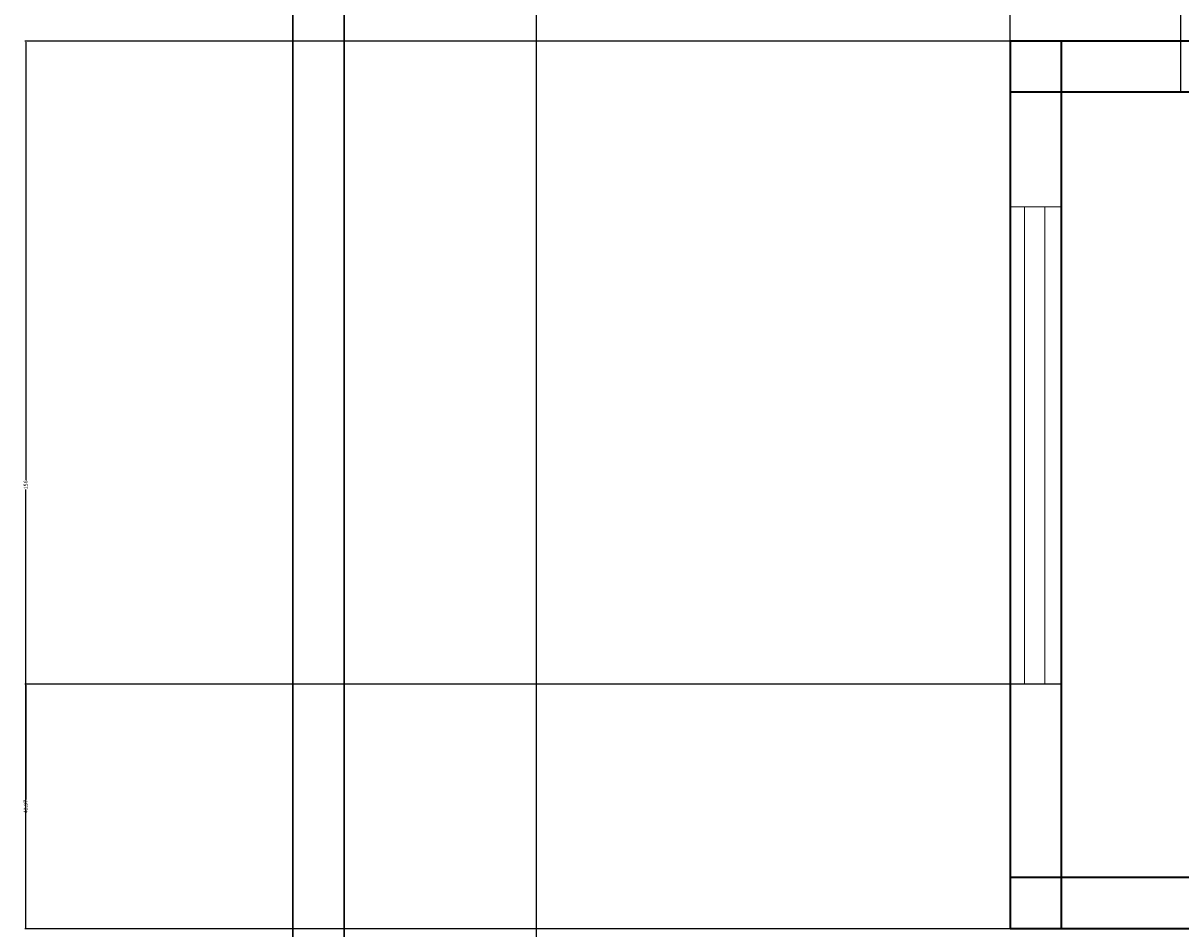
# Model space of a CAD drawing. Units: inches. Extents: x 867 to 1667, y -234 to 788.
# Tile 26 of 42: x 867 to 1071, y 258 to 417. Entities that reach past the tile are written whole.
import ezdxf

# ---------------------------------------------------------------- set-up
doc = ezdxf.new("R2010")
doc.units = ezdxf.units.IN
doc.header["$MEASUREMENT"] = 0
for name, color, linetype, lineweight in [('A-ANNO-DIMS', 2, 'Continuous', 18), ('A-Glaz', 92, 'Continuous', 18), ('A-Wall', 7, 'Continuous', 35), ('A-WALL-SITE', 8, 'Continuous', 30)]:
    doc.layers.add(name, color=color, linetype=linetype, lineweight=lineweight)
doc.styles.get("Standard").update_dxf_attribs({"font": 'arial.ttf'})
doc.dimstyles.get("Standard").update_dxf_attribs({"dimtxt": 0.6875, "dimasz": 0.18, "dimexe": 0.18, "dimexo": 0.0625, "dimgap": 0.09, "dimtad": 0, "dimdec": 4, "dimzin": 0, "dimdsep": 46, "dimlunit": 4, "dimtxsty": 'Standard', "dimcen": 0.09, "dimadec": 0, "dimazin": 0, "dimtfac": 1, "dimtdec": 4, "dimtofl": 0, "dimtmove": 0, "dimatfit": 3, "dimfxl": 1, "dimtolj": 1, "dimtzin": 0, "dimarcsym": 0})

# ---------------------------------------------------------------- blocks, each defined once
blk = doc.blocks.new('WIN-83_90IN')
for p, q in [((0, 83.9), (9, 83.9)), ((2.51, 83.9), (2.51, 0)), ((6.08, 0), (6.08, 83.9)), ((0, 0), (9, 0))]:
    blk.add_line(p, q)
blk = doc.blocks.new('*D28')
at = {"layer": 'A-ANNO-DIMS', "color": 0, "lineweight": -2, "transparency": 16777216}
for p, q in [((914.89, 623.55), (914.89, -233.54)), ((957.64, 623.55), (957.64, -233.54)), ((915.07, -233.36), (935, -233.36)), ((957.46, -233.36), (937.53, -233.36))]:
    blk.add_line(p, q, dxfattribs=at)
at = {"layer": 'A-ANNO-DIMS', "color": 0, "transparency": 16777216}
for points in [[(915.07, -233.33), (915.07, -233.39), (914.89, -233.36)], [(957.46, -233.33), (957.46, -233.39), (957.64, -233.36)]]:
    blk.add_solid(points, dxfattribs=at)
at = {"layer": 'Defpoints', "color": 0, "transparency": 16777216}
for p in [(914.89, 623.62), (957.64, 623.62), (914.89, -233.36)]:
    blk.add_point(p, dxfattribs=at)
at = {"layer": 'A-ANNO-DIMS', "color": 0, "transparency": 16777216, "insert": (936.26, -233.36), "char_height": 0.688, "attachment_point": 5}
blk.add_mtext('\\A1;42.75', dxfattribs=at)
blk = doc.blocks.new('*D35')
at = {"layer": 'A-ANNO-DIMS', "color": 0, "lineweight": -2, "transparency": 16777216}
for p, q in [((1040.89, 413.68), (1040.89, 787.75)), ((1041.07, 787.57), (1055.31, 787.57)), ((1070.71, 787.57), (1056.47, 787.57)), ((1070.89, 404.68), (1070.89, 787.75))]:
    blk.add_line(p, q, dxfattribs=at)
at = {"layer": 'A-ANNO-DIMS', "color": 0, "transparency": 16777216}
for points in [[(1041.07, 787.6), (1041.07, 787.54), (1040.89, 787.57)], [(1070.71, 787.6), (1070.71, 787.54), (1070.89, 787.57)]]:
    blk.add_solid(points, dxfattribs=at)
at = {"layer": 'Defpoints', "color": 0, "transparency": 16777216}
for p in [(1070.89, 787.57), (1040.89, 413.62), (1070.89, 404.62)]:
    blk.add_point(p, dxfattribs=at)
at = {"layer": 'A-ANNO-DIMS', "color": 0, "transparency": 16777216, "insert": (1055.89, 787.57), "char_height": 0.688, "attachment_point": 5}
blk.add_mtext('\\A1;30', dxfattribs=at)
blk = doc.blocks.new('*D39')
at = {"layer": 'A-ANNO-DIMS', "color": 0, "lineweight": -2, "transparency": 16777216}
for p, q in [((1040.82, 413.62), (867.76, 413.62)), ((867.94, 413.44), (867.94, 336.43)), ((867.94, 257.8), (867.94, 334.8)), ((1040.82, 257.62), (867.76, 257.62))]:
    blk.add_line(p, q, dxfattribs=at)
at = {"layer": 'A-ANNO-DIMS', "color": 0, "transparency": 16777216}
for points in [[(867.91, 413.44), (867.97, 413.44), (867.94, 413.62)], [(867.91, 257.8), (867.97, 257.8), (867.94, 257.62)]]:
    blk.add_solid(points, dxfattribs=at)
at = {"layer": 'Defpoints', "color": 0, "transparency": 16777216}
for p in [(867.94, 413.62), (1040.89, 413.62), (1040.89, 257.62)]:
    blk.add_point(p, dxfattribs=at)
at = {"layer": 'A-ANNO-DIMS', "color": 0, "transparency": 16777216, "insert": (867.94, 335.62), "char_height": 0.688, "attachment_point": 5, "rotation": 90}
blk.add_mtext('\\A1;156', dxfattribs=at)
blk = doc.blocks.new('*D56')
at = {"layer": 'A-ANNO-DIMS', "color": 0, "lineweight": -2, "transparency": 16777216}
for p, q in [((1049.82, 300.59), (867.76, 300.59)), ((867.94, 300.41), (867.94, 280.37)), ((867.94, 257.8), (867.94, 277.84)), ((1049.82, 257.62), (867.76, 257.62))]:
    blk.add_line(p, q, dxfattribs=at)
at = {"layer": 'A-ANNO-DIMS', "color": 0, "transparency": 16777216}
for points in [[(867.91, 300.41), (867.97, 300.41), (867.94, 300.59)], [(867.91, 257.8), (867.97, 257.8), (867.94, 257.62)]]:
    blk.add_solid(points, dxfattribs=at)
at = {"layer": 'Defpoints', "color": 0, "transparency": 16777216}
for p in [(867.94, 300.59), (1049.89, 300.59), (1049.89, 257.62)]:
    blk.add_point(p, dxfattribs=at)
at = {"layer": 'A-ANNO-DIMS', "color": 0, "transparency": 16777216, "insert": (867.94, 279.1), "char_height": 0.688, "attachment_point": 5, "rotation": 90}
blk.add_mtext('\\A1;42.97', dxfattribs=at)

msp = doc.modelspace()

# ---------------------------------------------------------------- linework, layer by layer
at = {"layer": 'A-Wall'}
for p, q in [((1040.8866, 413.617), (1040.8866, 257.617)), ((1529.8866, 413.617), (1040.8866, 413.617)), ((1049.8866, 413.617), (1049.8866, 257.617)), ((1559.8866, 404.617), (1040.8866, 404.617)), ((1160.8866, 266.617), (1040.8866, 266.617)), ((1160.8866, 257.617), (1040.8866, 257.617))]:
    msp.add_line(p, q, dxfattribs=at)
at = {"layer": 'A-WALL-SITE'}
for p, q in [((914.8866, 740.617), (914.8866, -186.4081)), ((923.8866, 740.617), (923.8866, -186.4081))]:
    msp.add_line(p, q, dxfattribs=at)

# ---------------------------------------------------------------- block references
at = {"layer": 'A-Glaz'}
msp.add_blockref('WIN-83_90IN', (1040.887, 300.5855), dxfattribs=at)

# ---------------------------------------------------------------- dimensions: what is measured, and where the dimension line sits
at = {"layer": 'A-ANNO-DIMS'}
for base, p1, p2, override, picture, middle in [((1070.8866, 787.567), (1040.8866, 413.617), (1070.8866, 404.617), {"dimdec": 0, "dimlfac": 1, "dimrnd": 0, "dimzin": 0, "dimdsep": 46, "dimlunit": 2}, '*D35', (1055.8866, 787.567)), ((914.8866, -233.3581), (957.6375, 623.617), (914.8866, 623.617), {"dimdec": 2, "dimlfac": 1, "dimrnd": 0, "dimzin": 0, "dimdsep": 46, "dimlunit": 2}, '*D28', (936.2621, -233.3581))]:
    dim = msp.add_linear_dim(base=base, p1=p1, p2=p2, dimstyle='Standard', override=override, dxfattribs=at)
    dim.commit()
    dim.dimension.update_dxf_attribs({"geometry": picture, "text_midpoint": middle})
for base, p1, p2, override, picture, middle in [((867.9366, 413.617), (1040.8866, 257.617), (1040.8866, 413.617), {"dimdec": 0, "dimlfac": 1, "dimrnd": 0, "dimzin": 0, "dimdsep": 46, "dimlunit": 2}, '*D39', (867.9366, 335.617)), ((867.9366, 300.5856), (1049.8866, 257.617), (1049.8866, 300.5856), {"dimdec": 2, "dimlfac": 1, "dimrnd": 0, "dimzin": 0, "dimdsep": 46, "dimlunit": 2}, '*D56', (867.9366, 279.1013))]:
    dim = msp.add_linear_dim(base=base, p1=p1, p2=p2, angle=90, dimstyle='Standard', override=override, dxfattribs=at)
    dim.commit()
    dim.dimension.update_dxf_attribs({"geometry": picture, "text_midpoint": middle})

doc.saveas('drawing.dxf')
